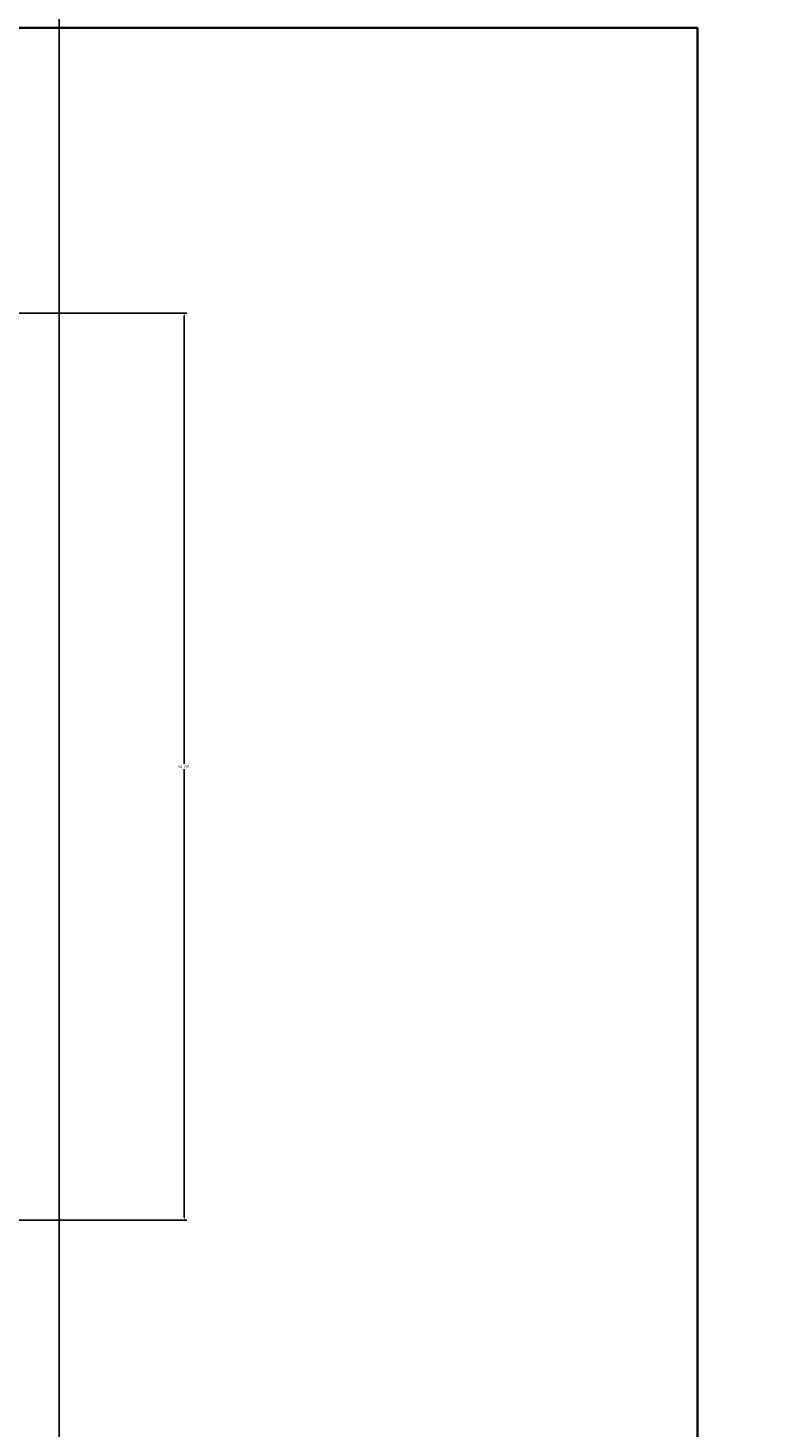
# Model space of a CAD drawing. Units: inches. Extents: x -61 to 1599, y -1316 to 257.
# Tile 152 of 204: x 490 to 540, y 52 to 149. Entities that reach past the tile are written whole.
import ezdxf

# ---------------------------------------------------------------- set-up
doc = ezdxf.new("R2010")
doc.units = ezdxf.units.IN
doc.header["$MEASUREMENT"] = 0
doc.layers.add('A-ANNO-DIMS', color=2, linetype='Continuous', lineweight=18)
doc.layers.add('WALLS', color=4, linetype='Continuous', lineweight=35)
doc.styles.get("Standard").update_dxf_attribs({"font": 'arial.ttf'})
doc.dimstyles.get("Standard").update_dxf_attribs({"dimtxt": 0.18, "dimasz": 0.18, "dimexe": 0.18, "dimexo": 0.0625, "dimgap": 0.09, "dimtad": 0, "dimtih": 1, "dimtoh": 1, "dimdec": 0, "dimzin": 0, "dimdsep": 46, "dimlunit": 3, "dimtxsty": 'Standard', "dimcen": 0.09, "dimadec": 0, "dimazin": 0, "dimtfac": 1, "dimtdec": 0, "dimtofl": 0, "dimtmove": 0, "dimatfit": 3, "dimfxl": 1, "dimtolj": 1, "dimtzin": 0, "dimarcsym": 0})

# ---------------------------------------------------------------- blocks, each defined once
blk = doc.blocks.new('*D677')
at = {"layer": 'A-ANNO-DIMS', "color": 0, "lineweight": -2, "transparency": 16777216}
for p, q in [((488.407, 129.084), (500.607, 129.084)), ((500.427, 128.904), (500.427, 98.089)), ((500.427, 66.909), (500.427, 97.725)), ((488.407, 66.729), (500.607, 66.729))]:
    blk.add_line(p, q, dxfattribs=at)
at = {"layer": 'A-ANNO-DIMS', "color": 0, "transparency": 16777216}
for points in [[(500.397, 128.904), (500.457, 128.904), (500.427, 129.084)], [(500.397, 66.909), (500.457, 66.909), (500.427, 66.729)]]:
    blk.add_solid(points, dxfattribs=at)
at = {"layer": 'DEFPOINTS', "color": 0, "transparency": 16777216}
for p in [(488.345, 129.084), (500.427, 129.084), (488.345, 66.729)]:
    blk.add_point(p, dxfattribs=at)
at = {"layer": 'A-ANNO-DIMS', "color": 0, "transparency": 16777216, "insert": (500.427, 97.907), "char_height": 0.18, "attachment_point": 5}
blk.add_mtext('\\A1;62 TYP.', dxfattribs=at)
blk = doc.blocks.new('*D704')
at = {"layer": 'A-ANNO-DIMS', "color": 0, "lineweight": -2, "transparency": 16777216}
for p, q in [((491.833, -616.882), (491.833, 257.457)), ((492.013, 257.277), (517.874, 257.277)), ((544.523, 257.277), (518.661, 257.277)), ((544.703, -616.882), (544.703, 257.457))]:
    blk.add_line(p, q, dxfattribs=at)
at = {"layer": 'A-ANNO-DIMS', "color": 0, "transparency": 16777216}
for points in [[(492.013, 257.307), (492.013, 257.247), (491.833, 257.277)], [(544.523, 257.307), (544.523, 257.247), (544.703, 257.277)]]:
    blk.add_solid(points, dxfattribs=at)
at = {"layer": 'DEFPOINTS', "color": 0, "transparency": 16777216}
for p in [(544.703, 257.277), (491.833, -616.945), (544.703, -616.945)]:
    blk.add_point(p, dxfattribs=at)
at = {"layer": 'A-ANNO-DIMS', "color": 0, "transparency": 16777216, "insert": (518.268, 257.277), "char_height": 0.18, "attachment_point": 5}
blk.add_mtext('\\A1;52.87', dxfattribs=at)

msp = doc.modelspace()

# ---------------------------------------------------------------- linework, layer by layer
at = {"layer": 'WALLS'}
for p, q in [((403.7028, 148.6771), (535.7028, 148.6771)), ((535.7028, 148.6771), (535.7028, -7.3229))]:
    msp.add_line(p, q, dxfattribs=at)

# ---------------------------------------------------------------- dimensions: what is measured, and where the dimension line sits
at = {"layer": 'A-ANNO-DIMS'}
dim = msp.add_linear_dim(base=(544.7028, 257.2771), p1=(491.8327, -616.9446), p2=(544.7028, -616.9446), dimstyle='Standard', override={"dimdec": 2, "dimlfac": 1, "dimrnd": 0, "dimzin": 0, "dimdsep": 46, "dimlunit": 2}, dxfattribs=at)
dim.commit()
dim.dimension.update_dxf_attribs({"geometry": '*D704', "text_midpoint": (518.2677, 257.2771)})
dim = msp.add_linear_dim(base=(500.4274, 129.084), p1=(488.3448, 66.7295), p2=(488.3448, 129.084), angle=90, text='<> TYP.', dimstyle='Standard', override={"dimdec": 0, "dimlfac": 1, "dimrnd": 0, "dimzin": 0, "dimdsep": 46, "dimlunit": 2}, dxfattribs=at)
dim.commit()
dim.dimension.update_dxf_attribs({"geometry": '*D677', "text_midpoint": (500.4274, 97.9068)})

doc.saveas('drawing.dxf')
